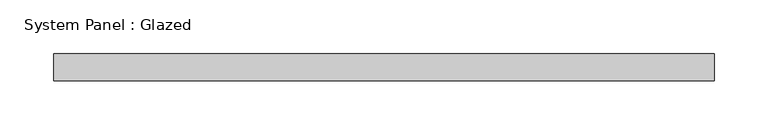
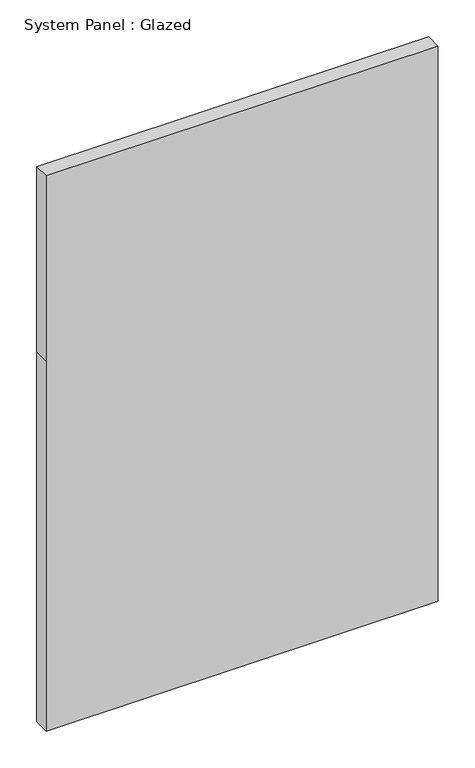
"""IFC4 building model written with IfcOpenShell, lengths in millimetres: plate geometry, System Panel : Glazed."""

from ifc_helpers import new_model, si_unit, frame, origin, place, context, project, spatial, polyline, outline, extrude, source, transform, mapped, element, save


def system_panel_glazed_3f50d1a2(model_context):
    return source(origin(), model_context, "Body", "SweptSolid", [
        extrude(outline(polyline([(0.0, -307.975), (0.0, 307.975), (614.4496655, 307.975), (921.6744982, 307.975), (921.6744982, -307.975), (614.4496655, -307.975), (0.0, -307.975)])), frame((0.0, 19.05, 0.0), z_axis=(0.0, 1.0, 0.0), x_axis=(0.0, 0.0, 1.0)), (0.0, 0.0, 1.0), 25.4),
    ])


if __name__ == "__main__":
    model = new_model("IFC4")
    model_context = context("Model", 3, world=origin())
    ifc_project = project(units=[si_unit("LENGTHUNIT", "METRE", prefix="MILLI")], contexts=[model_context])
    site = spatial("IfcSite", under=ifc_project)
    building = spatial("IfcBuilding", under=site)
    placement = place(None, origin())
    system_panel_glazed_shape = system_panel_glazed_3f50d1a2(model_context)
    element("IfcPlate", 1, ObjectType="System Panel : Glazed", at=placement, inside=building, context=model_context, shape_type="MappedRepresentation", body=[
        mapped(system_panel_glazed_shape, transform((0.0, 0.0, 0.0), x_axis=(1.0, 0.0, 0.0), y_axis=(0.0, 1.0, 0.0), z_axis=(0.0, 0.0, 1.0))),
    ])
    save(model, "model.ifc")

# Revit data of these elements
# Type "System Panel : Glazed"
#   Construction Type Id = "GSP4R"
#   Analytic Construction = "1/8 in Pilkington single glazing"
#   Visual Light Transmittance = 0.9
#   Solar Heat Gain Coefficient = 0.86
#   Heat Transfer Coefficient (U) = 1.18115 BTU/(h·ft²·°F)
#   Define Thermal Properties by = 1
# Element 1 (IfcPlate, "System Panel : Glazed")
#   Materials on its faces: "Glass"
# Materials
#   "Glass": class "Glass", colour RGB 0 128 192, transparency 0.75, Description = "Soda Lime Glass", Cost = 0
